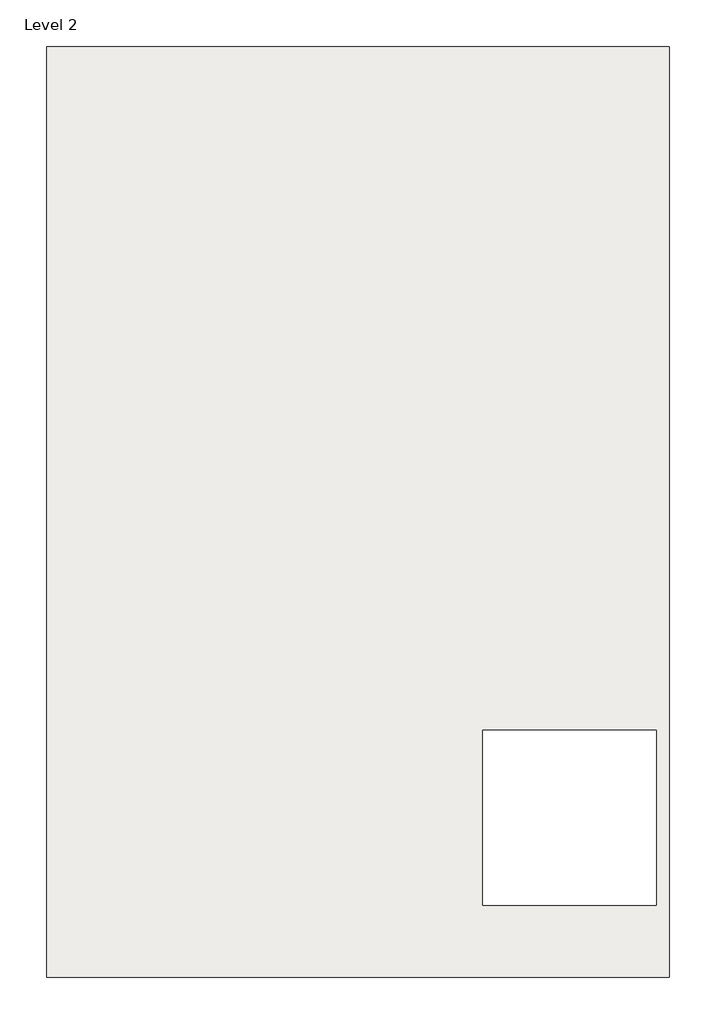
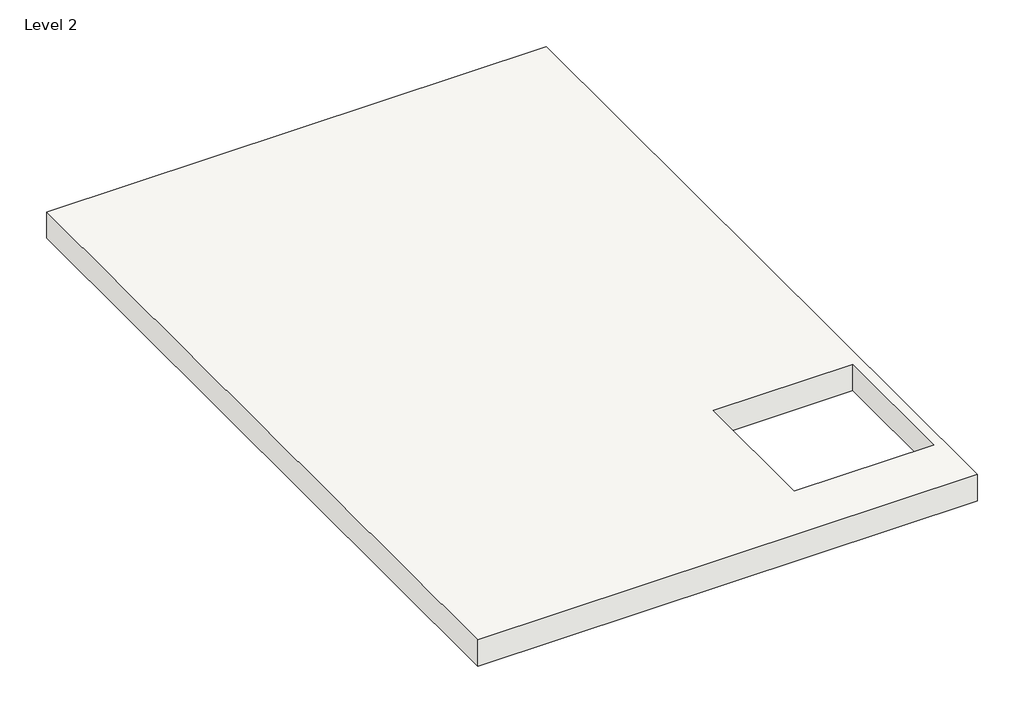
# One storey: 1 roof.
"""IFC4 building model written with IfcOpenShell, lengths in millimetres."""

from ifc_helpers import new_model, si_unit, frame, origin, place, context, project, spatial, polyline, outline, extrude, element, save

model = new_model("IFC4")

# Units and contexts
model_context = context("Model", 3, world=origin())
ifc_project = project(units=[si_unit("LENGTHUNIT", "METRE", prefix="MILLI")], contexts=[model_context])

# Site, building, storey
site = spatial("IfcSite", under=ifc_project)
building = spatial("IfcBuilding", under=site)
storey = spatial("IfcBuildingStorey", under=building, Name="Level 2", Elevation=3048.0)

# Roof
placement = place(None, origin())
element("IfcRoof", 1, ObjectType="Steel Truss - Insulation on Metal Deck - EPDM", at=placement, inside=storey, context=model_context, shape_type="SweptSolid", body=[
    extrude(outline(polyline([(-12218.8047602, 13434.9174997), (-2363.6047602, 13434.9174997), (-2363.6047602, -1297.0825003), (-12218.8047602, -1297.0825003), (-12218.8047602, 13434.9174997)]), holes=[polyline([(-5318.5510787, 2614.5174997), (-5318.5510787, -154.0825003), (-2566.8047602, -154.0825003), (-2566.8047602, 2614.5174997), (-5318.5510787, 2614.5174997)])]), frame((0.0, 0.0, 3048.0), z_axis=(0.0, 0.0, 1.0), x_axis=(1.0, 0.0, 0.0)), (0.0, 0.0, 1.0), 546.1),
])

save(model, "model.ifc")

# Revit data of these elements
# Type "Steel Truss - Insulation on Metal Deck - EPDM"
#   Assembly Code = "B1020"
#   Layers, outside or top first: 0' - 0 1/4" "Roofing, EPDM Membrane" (function 4); 0' - 5" "Rigid insulation" (function 3); 0' - 0 1/4" "Metal Deck" (function 1); 1' - 4" "Structure, Steel Bar Joist Layer" (function 1)
# Element 1 (IfcRoof, "Steel Truss - Insulation on Metal Deck - EPDM")
#   built-in parameter 1001705 = 11.7917 (stored number, unit not read)
#   built-in parameter 1001710 = 33615
#   Phase Created = New Construction
#   Materials on its faces: "Structure, Steel Bar Joist Layer", "Roofing, EPDM Membrane"
# Materials
#   "Roofing, EPDM Membrane": class "Generic", colour RGB 127 127 127, transparency 0, Description = "EPDM roof membrane", Cost = 0
#   "Rigid insulation": class "Generic", colour RGB 127 127 127, transparency 0, Description = "Rigid foam insulation board", Cost = 0
#   "Metal Deck": class "Metal", colour RGB 199 199 199, transparency 0, Description = "Steel, mill finish", Cost = 0
#   "Structure, Steel Bar Joist Layer": class "Metal", colour RGB 127 127 127, transparency 0, Description = "Bar joists, thermal airspace", Cost = 0
